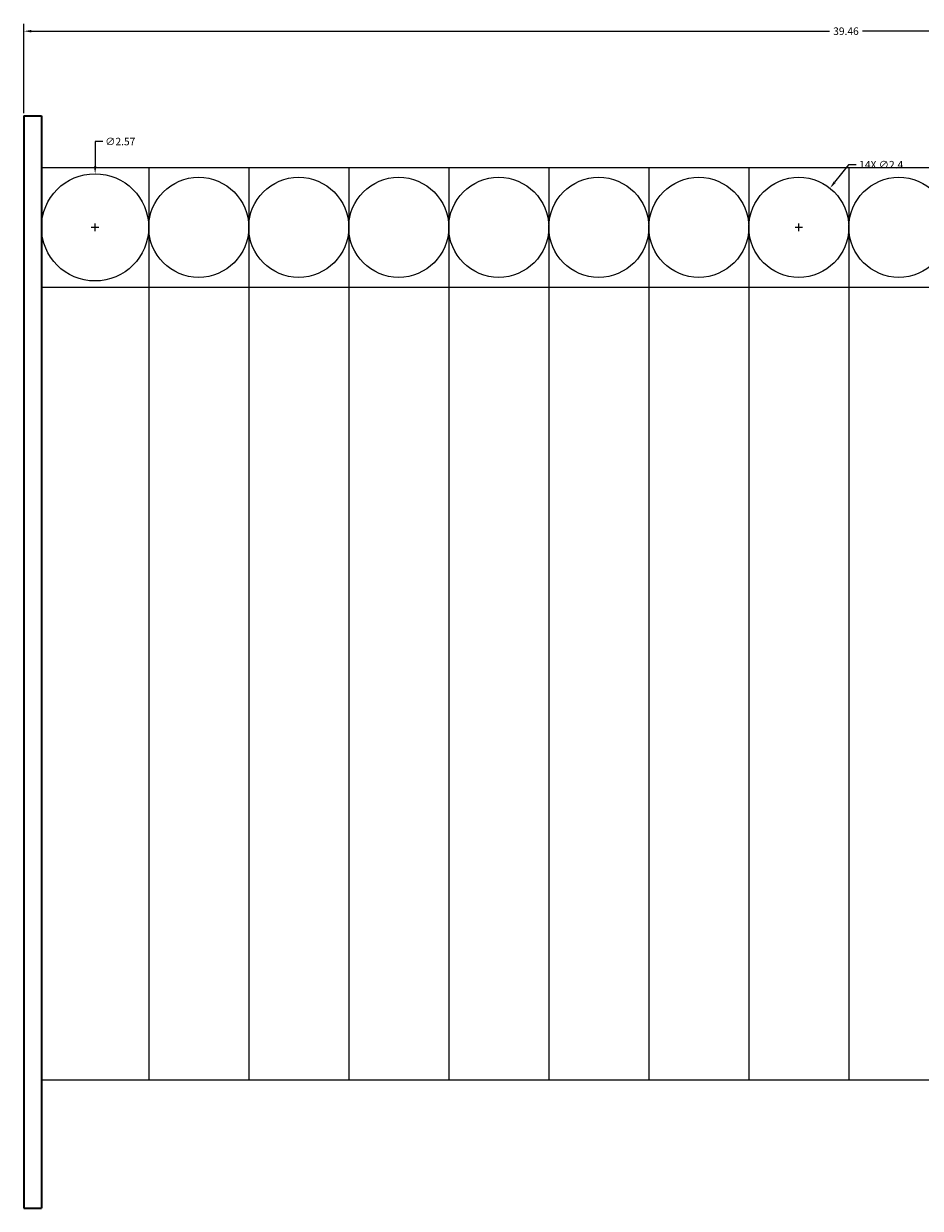
# Model space of a CAD drawing. Units: inches. Extents: x 756 to 915, y 488 to 695.
# Tile 8 of 25: x 866 to 888, y 513 to 541. Entities that reach past the tile are written whole.
import ezdxf

# ---------------------------------------------------------------- set-up
doc = ezdxf.new("R2010")
doc.units = ezdxf.units.IN
doc.header["$MEASUREMENT"] = 0
for name, color, linetype, lineweight in [('L-FENC-PCKT', 7, 'Continuous', 18), ('L-FENC-POST', 7, 'Continuous', 35), ('L-FENC-RAIL', 7, 'Continuous', 25), ('L-FENC-RING', 7, 'Continuous', 18), ('M-DIMS', 2, 'Continuous', 18)]:
    doc.layers.add(name, color=color, linetype=linetype, lineweight=lineweight)
doc.styles.get("Standard").update_dxf_attribs({"font": 'arial.ttf'})
doc.dimstyles.get("Standard").update_dxf_attribs({"dimtxt": 0.18, "dimasz": 0.18, "dimexe": 0.18, "dimexo": 0.0625, "dimgap": 0.09, "dimtad": 0, "dimtih": 1, "dimtoh": 1, "dimdec": 0, "dimzin": 0, "dimdsep": 46, "dimlunit": 3, "dimtxsty": 'Standard', "dimcen": 0.09, "dimadec": 0, "dimazin": 0, "dimtfac": 1, "dimtdec": 0, "dimtofl": 0, "dimtmove": 0, "dimatfit": 3, "dimfxl": 1, "dimtolj": 1, "dimtzin": 0, "dimarcsym": 0})

# ---------------------------------------------------------------- blocks, each defined once
blk = doc.blocks.new('FENCE-POST-LEFT')
for p, q in [((0, 26.207), (0, 0)), ((0, 26.207), (0.426, 26.207)), ((0.426, 26.207), (0.426, 0)), ((0.426, 26.207), (0.426, 0)), ((0, 0), (0.426, 0))]:
    blk.add_line(p, q)
blk = doc.blocks.new('FENCE-PLUS-RING-BAND')
for centre, radius in [((1.286, 1.286), 1.286), ((3.773, 1.286), 1.2), ((6.173, 1.286), 1.2), ((8.572, 1.286), 1.2), ((10.972, 1.286), 1.2), ((13.372, 1.286), 1.2), ((15.772, 1.286), 1.2), ((18.172, 1.286), 1.2), ((20.572, 1.286), 1.2), ((22.972, 1.286), 1.2), ((25.372, 1.286), 1.2), ((27.772, 1.286), 1.2), ((30.172, 1.286), 1.2), ((32.572, 1.286), 1.2), ((34.971, 1.286), 1.2), ((37.388, 1.286), 1.217)]:
    blk.add_circle(centre, radius)
blk = doc.blocks.new('*D63')
at = {"layer": 'Defpoints', "color": 0, "transparency": 16777216}
for p in [(905.684, 541.143), (866.226, 539.113), (905.684, 539.113)]:
    blk.add_point(p, dxfattribs=at)
at = {"layer": 'M-DIMS', "color": 0, "lineweight": -2, "transparency": 16777216}
for p, q in [((866.226, 539.175), (866.226, 541.323)), ((866.406, 541.143), (885.561, 541.143)), ((905.504, 541.143), (886.348, 541.143)), ((905.684, 539.175), (905.684, 541.323))]:
    blk.add_line(p, q, dxfattribs=at)
at = {"layer": 'M-DIMS', "color": 0, "transparency": 16777216}
for points in [[(866.406, 541.173), (866.406, 541.113), (866.226, 541.143)], [(905.504, 541.173), (905.504, 541.113), (905.684, 541.143)]]:
    blk.add_solid(points, dxfattribs=at)
at = {"layer": 'M-DIMS', "color": 0, "transparency": 16777216, "insert": (885.955, 541.143), "char_height": 0.18, "attachment_point": 5}
blk.add_mtext('\\A1;39.46', dxfattribs=at)
blk = doc.blocks.new('*D81')
at = {"layer": 'Defpoints', "color": 0, "transparency": 16777216}
for p in [(867.94, 537.724), (867.937, 535.152)]:
    blk.add_point(p, dxfattribs=at)
at = {"layer": 'M-DIMS', "color": 0, "lineweight": -2, "transparency": 16777216}
for p, q in [((867.941, 538.496), (867.94, 537.904)), ((868.121, 538.496), (867.941, 538.496)), ((867.938, 536.348), (867.938, 536.528)), ((867.848, 536.438), (868.028, 536.438))]:
    blk.add_line(p, q, dxfattribs=at)
at = {"layer": 'M-DIMS', "color": 0, "transparency": 16777216}
blk.add_solid([(867.91, 537.904), (867.97, 537.904), (867.94, 537.724)], dxfattribs=at)
at = {"layer": 'M-DIMS', "color": 0, "transparency": 16777216, "insert": (868.543, 538.496), "char_height": 0.18, "attachment_point": 5}
blk.add_mtext('\\A1;∅2.57', dxfattribs=at)
blk = doc.blocks.new('*D82')
at = {"layer": 'Defpoints', "color": 0, "transparency": 16777216}
for p in [(885.571, 537.377), (884.077, 535.499)]:
    blk.add_point(p, dxfattribs=at)
at = {"layer": 'M-DIMS', "color": 0, "lineweight": -2, "transparency": 16777216}
for p, q in [((886.019, 537.941), (885.683, 537.518)), ((886.199, 537.941), (886.019, 537.941)), ((884.824, 536.348), (884.824, 536.528)), ((884.734, 536.438), (884.914, 536.438))]:
    blk.add_line(p, q, dxfattribs=at)
at = {"layer": 'M-DIMS', "color": 0, "transparency": 16777216}
blk.add_solid([(885.659, 537.537), (885.706, 537.499), (885.571, 537.377)], dxfattribs=at)
at = {"layer": 'M-DIMS', "color": 0, "transparency": 16777216, "insert": (886.8, 537.941), "char_height": 0.18, "attachment_point": 5}
blk.add_mtext('\\A1;14X ∅2.4', dxfattribs=at)

msp = doc.modelspace()

# ---------------------------------------------------------------- linework, layer by layer
at = {"layer": 'L-FENC-PCKT'}
for p, q in [((869.2247, 537.87), (869.2247, 515.9878)), ((871.6246, 537.87), (871.6246, 515.9878)), ((874.0245, 537.87), (874.0245, 515.9878)), ((876.4244, 537.87), (876.4244, 515.9878)), ((878.8243, 537.87), (878.8243, 515.9878)), ((881.2242, 537.87), (881.2242, 515.9878)), ((883.6241, 537.87), (883.6241, 515.9878)), ((886.024, 537.87), (886.024, 515.9878))]:
    msp.add_line(p, q, dxfattribs=at)
at = {"layer": 'L-FENC-RAIL'}
for p, q in [((866.6522, 537.87), (905.257, 537.87)), ((866.6522, 535.0056), (905.257, 535.0056)), ((866.6522, 515.9878), (905.257, 515.9878))]:
    msp.add_line(p, q, dxfattribs=at)

# ---------------------------------------------------------------- block references
at = {"layer": 'L-FENC-POST'}
msp.add_blockref('FENCE-POST-LEFT', (866.2259, 512.9061), dxfattribs=at)
at = {"layer": 'L-FENC-RING'}
msp.add_blockref('FENCE-PLUS-RING-BAND', (866.652, 535.1518), dxfattribs=at)

# ---------------------------------------------------------------- dimensions: what is measured, and where the dimension line sits
at = {"layer": 'M-DIMS'}
dim = msp.add_linear_dim(base=(905.6837, 541.1429), p1=(866.2255, 539.1129), p2=(905.6837, 539.1129), dimstyle='Standard', override={"dimdec": 2, "dimlfac": 1, "dimrnd": 0, "dimzin": 0, "dimdsep": 46, "dimlunit": 2}, dxfattribs=at)
dim.commit()
dim.dimension.update_dxf_attribs({"geometry": '*D63', "text_midpoint": (885.9546, 541.1429)})
dim = msp.add_diameter_dim_2p(p1=(867.9368, 535.1516), p2=(867.94, 537.724), dimstyle='Standard', override={"dimdec": 2, "dimlfac": 1, "dimrnd": 0, "dimzin": 0, "dimdsep": 46, "dimlunit": 2}, dxfattribs=at)
dim.commit()
dim.dimension.update_dxf_attribs({"geometry": '*D81', "text_midpoint": (868.5427, 538.4958), "dimtype": 163})
dim = msp.add_diameter_dim_2p(p1=(884.0772, 535.4986), p2=(885.5709, 537.377), text='14X <>', dimstyle='Standard', override={"dimdec": 1, "dimlfac": 1, "dimrnd": 0, "dimzin": 0, "dimdsep": 46, "dimlunit": 2}, dxfattribs=at)
dim.commit()
dim.dimension.update_dxf_attribs({"geometry": '*D82', "text_midpoint": (886.8005, 537.9406), "dimtype": 163})

doc.saveas('drawing.dxf')
